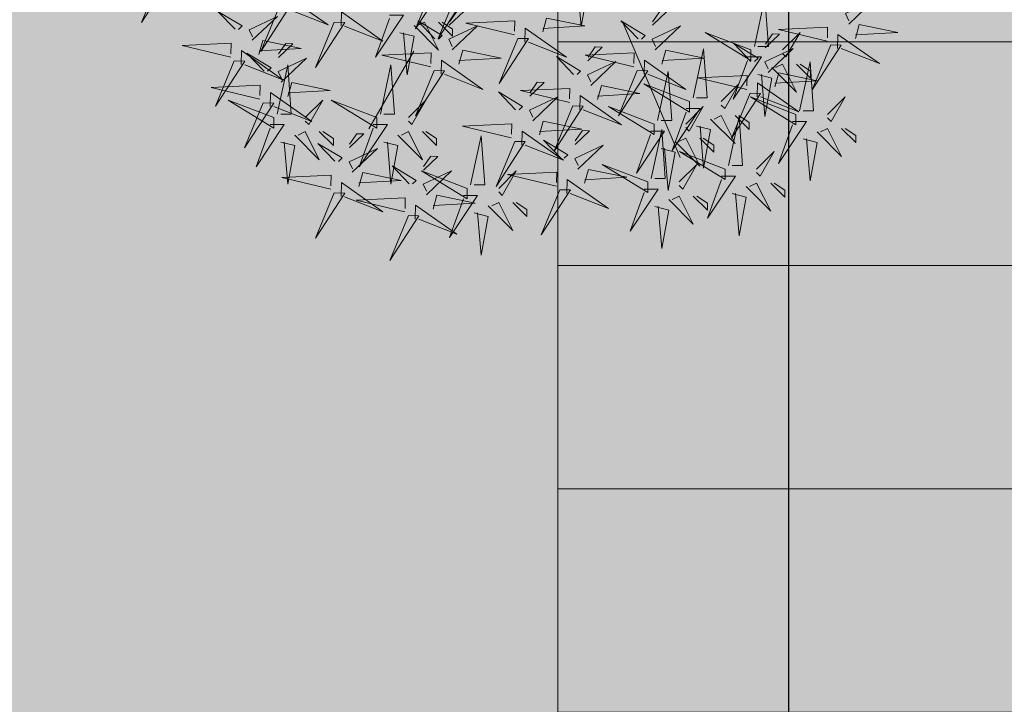
# Model space of a CAD drawing. Units: inches. Extents: x 1704 to 6393, y -157 to 1172.
# Tile 80 of 122: x 2048 to 2081, y 983 to 1006. Entities that reach past the tile are written whole.
import ezdxf

# ---------------------------------------------------------------- set-up
doc = ezdxf.new("R2010")
doc.units = ezdxf.units.IN
doc.header["$MEASUREMENT"] = 0
for name, color, linetype, lineweight in [('A-ANNO-DIMS', 7, 'Continuous', 13), ('L-DECK-PLNK-PATT', 250, 'Continuous', 13), ('L-HRDS', 8, 'Continuous', 18), ('L-shrub', 74, 'Continuous', 18)]:
    doc.layers.add(name, color=color, linetype=linetype, lineweight=lineweight)
doc.layers.add('L-DECK-PATT', color=35, linetype='Continuous', lineweight=13, true_color=0xa6725b)
doc.layers.add('L-HRDS-PATT', color=9, linetype='Continuous', lineweight=13, true_color=0xc5c1ba)
doc.styles.get("Standard").update_dxf_attribs({"font": 'arial.ttf'})
doc.dimstyles.get("Standard").update_dxf_attribs({"dimtxt": 6, "dimasz": 2, "dimexe": 0.18, "dimexo": 0.0625, "dimgap": 0.09, "dimtad": 0, "dimtih": 1, "dimtoh": 1, "dimdec": 1, "dimzin": 0, "dimdsep": 46, "dimlunit": 3, "dimtxsty": 'Standard', "dimblk": 'ARCHTICK', "dimcen": 0.09, "dimadec": 0, "dimazin": 0, "dimtfac": 1, "dimtdec": 1, "dimtofl": 0, "dimtmove": 0, "dimatfit": 3, "dimfxl": 1, "dimtolj": 1, "dimtzin": 0, "dimarcsym": 0})

# ---------------------------------------------------------------- blocks, each defined once
blk = doc.blocks.new('shrub3')
for p, q in [((-68.47, 143.52), (-106.19, 232.32)), ((68.94, 162.35), (98.58, 213.48))]:
    blk.add_line(p, q)
for points in [[(72.58, 270.39), (84.86, 300.11), (65.67, 270.57), (72.58, 270.39)], [(-89.4, 264.53), (-98.64, 266.83), (-94.02, 292.2), (-91.71, 264.53)], [(29.32, 268.76), (20.08, 271.07), (24.7, 296.43), (27.01, 268.76)], [(36.24, 257.23), (27.01, 257.23), (45.48, 284.9), (36.24, 259.54)], [(121.34, 255.57), (133.62, 285.29), (114.43, 255.75), (121.34, 255.57)], [(-140.28, 256.06), (-149.52, 258.36), (-144.9, 283.73), (-142.59, 256.06)], [(-82.48, 253), (-91.71, 253), (-73.24, 280.67), (-82.48, 255.31)], [(-27.06, 253.45), (-14.78, 283.17), (-33.97, 253.63), (-27.06, 253.45)], [(20.08, 264.15), (3.92, 280.29), (13.16, 261.85), (17.78, 264.15)], [(68.03, 272.82), (67.8, 263.59), (40.6, 282.74), (65.73, 272.87)], [(-133.36, 244.53), (-142.59, 244.53), (-124.12, 272.2), (-133.36, 246.84)], [(-98.64, 259.92), (-114.8, 276.06), (-105.56, 257.61), (-100.94, 259.92)], [(-149.52, 251.45), (-165.68, 267.59), (-156.44, 249.14), (-151.83, 251.45)], [(-114.8, 257.61), (-124.03, 266.83), (-124.03, 262.22), (-117.11, 257.61)], [(-31.61, 255.88), (-31.84, 246.65), (-59.04, 265.8), (-33.91, 255.94)], [(3.92, 261.85), (-5.31, 271.07), (-5.31, 266.46), (1.62, 261.85)], [(56.33, 266.18), (53.8, 257.01), (28.56, 262.26), (56.27, 263.87)], [(74.83, 268.03), (106.93, 260.3), (74.6, 258.8), (74.77, 265.72)], [(116.79, 258), (116.56, 248.76), (89.36, 267.92), (114.49, 258.05)], [(33.94, 252.62), (63.95, 241.09), (33.94, 259.54), (33.94, 252.62)], [(-165.68, 249.14), (-174.91, 258.36), (-174.91, 253.75), (-167.99, 249.14)], [(-105.56, 248.39), (-117.11, 236.86), (-107.87, 253), (-105.56, 250.69)], [(-93.64, 226.42), (-102.88, 228.72), (-98.26, 254.08), (-95.95, 226.42)], [(-84.78, 248.39), (-54.77, 236.86), (-84.78, 255.31), (-84.78, 248.39)], [(13.16, 252.62), (1.62, 241.09), (10.85, 257.23), (13.16, 254.93)], [(60.71, 256.84), (44.17, 241.08), (62.84, 249.85), (60.65, 254.53)], [(123.59, 253.21), (155.69, 245.48), (123.36, 243.97), (123.53, 250.9)], [(-186.92, 220.06), (-196.16, 222.37), (-191.54, 247.73), (-189.23, 220.06)], [(-135.66, 239.92), (-105.65, 228.39), (-135.66, 246.84), (-135.66, 239.92)], [(-87.09, 246.08), (-94.02, 213.8), (-96.33, 246.08), (-89.4, 246.08)], [(-43.31, 249.24), (-45.84, 240.07), (-71.08, 245.32), (-43.37, 246.93)], [(-24.81, 251.09), (7.29, 243.36), (-25.04, 241.86), (-24.87, 248.78)], [(2.62, 221.69), (14.9, 251.41), (-4.29, 221.87), (2.62, 221.69)], [(31.63, 250.32), (24.7, 218.04), (22.39, 250.32), (29.32, 250.32)], [(72.06, 249.62), (83.3, 237.79), (67.4, 247.43), (69.76, 249.68)], [(105.09, 251.36), (102.56, 242.19), (77.32, 247.44), (105.04, 249.05)], [(88.68, 222.18), (79.44, 224.49), (84.06, 249.85), (86.37, 222.18)], [(156.52, 222.18), (147.29, 224.49), (151.9, 249.85), (154.21, 222.18)], [(-156.44, 239.92), (-167.99, 228.39), (-158.75, 244.53), (-156.44, 242.22)], [(-86.72, 214.89), (-95.95, 214.89), (-77.48, 242.56), (-86.72, 217.19)], [(-38.93, 239.9), (-55.47, 224.14), (-36.8, 232.91), (-38.99, 237.59)], [(62.61, 240.62), (53.16, 231.62), (57.77, 231.51), (62.55, 238.31)], [(109.47, 242.01), (92.93, 226.26), (111.6, 235.03), (109.41, 239.71)], [(-180, 208.53), (-189.23, 208.53), (-170.76, 236.2), (-180, 210.84)], [(-137.97, 237.61), (-144.9, 205.33), (-147.21, 237.61), (-140.28, 237.61)], [(-116.96, 211.59), (-126.2, 213.9), (-121.58, 239.26), (-119.27, 211.59)], [(-102.88, 221.8), (-119.04, 237.94), (-109.8, 219.5), (-105.18, 221.8)], [(-1.93, 224.12), (-2.16, 214.89), (-29.36, 234.04), (-4.23, 224.17)], [(79.44, 217.57), (63.28, 233.71), (72.52, 215.26), (77.14, 217.57)], [(95.61, 210.65), (86.37, 210.65), (104.84, 238.32), (95.61, 212.96)], [(120.82, 234.8), (132.06, 222.97), (116.16, 232.61), (118.52, 234.86)], [(147.29, 217.57), (131.13, 233.71), (140.36, 215.26), (144.98, 217.57)], [(163.45, 210.65), (154.21, 210.65), (172.68, 238.32), (163.45, 212.96)], [(-196.16, 215.45), (-212.32, 231.59), (-203.08, 213.15), (-198.47, 215.45)], [(-119.04, 219.5), (-128.27, 228.72), (-128.27, 224.11), (-121.35, 219.5)], [(-110.04, 200.06), (-119.27, 200.06), (-100.8, 227.73), (-110.04, 202.37)], [(-35.54, 198.4), (-23.26, 228.12), (-42.45, 198.58), (-35.54, 198.4)], [(-27.58, 232.68), (-16.34, 220.86), (-32.24, 230.49), (-29.88, 232.74)], [(-212.32, 213.15), (-221.55, 222.37), (-221.55, 217.76), (-214.63, 213.15)], [(-126.2, 206.98), (-142.36, 223.12), (-133.12, 204.68), (-128.5, 206.98)], [(-37.03, 223.68), (-46.48, 214.68), (-41.87, 214.57), (-37.09, 221.37)], [(63.28, 215.26), (54.05, 224.49), (54.05, 219.87), (60.98, 215.26)], [(111.37, 225.8), (101.92, 216.8), (106.53, 216.68), (111.31, 223.49)], [(131.13, 215.26), (121.89, 224.49), (121.89, 219.87), (128.82, 215.26)], [(167.98, 196.29), (180.26, 226), (161.07, 196.46), (167.98, 196.29)], [(-152.14, 189.93), (-139.86, 219.65), (-159.05, 190.11), (-152.14, 189.93)], [(-142.36, 204.68), (-151.59, 213.9), (-151.59, 209.29), (-144.67, 204.68)], [(-109.8, 210.27), (-121.35, 198.75), (-112.11, 214.89), (-109.8, 212.58)], [(-89.02, 210.27), (-59.01, 198.75), (-89.02, 217.19), (-89.02, 210.27)], [(-13.63, 217.48), (-16.16, 208.31), (-41.4, 213.56), (-13.69, 215.17)], [(4.87, 219.33), (36.97, 211.6), (4.64, 210.1), (4.81, 217.02)], [(-203.08, 203.92), (-214.63, 192.39), (-205.39, 208.53), (-203.08, 206.23)], [(-182.31, 203.92), (-152.29, 192.39), (-182.31, 210.84), (-182.31, 203.92)], [(-91.33, 207.97), (-98.26, 175.69), (-100.57, 207.97), (-93.64, 207.97)], [(-40.09, 200.83), (-40.32, 191.59), (-67.52, 210.75), (-42.39, 200.88)], [(-9.25, 208.13), (-25.79, 192.38), (-7.12, 201.15), (-9.31, 205.83)], [(72.52, 206.04), (60.98, 194.51), (70.21, 210.65), (72.52, 208.35)], [(93.3, 206.04), (123.31, 194.51), (93.3, 212.96), (93.3, 206.04)], [(140.36, 206.04), (128.82, 194.51), (138.05, 210.65), (140.36, 208.35)], [(163.43, 198.71), (163.2, 189.48), (136, 208.63), (161.13, 198.77)], [(161.14, 206.04), (191.15, 194.51), (161.14, 212.96), (161.14, 206.04)], [(-184.61, 201.62), (-191.54, 169.34), (-193.85, 201.62), (-186.92, 201.62)], [(-156.69, 192.36), (-156.92, 183.12), (-184.12, 202.28), (-159, 192.41)], [(-157.24, 177.72), (-166.48, 180.02), (-161.86, 205.38), (-159.55, 177.72)], [(-112.34, 195.45), (-82.33, 183.92), (-112.34, 202.37), (-112.34, 195.45)], [(-77.94, 175.11), (-65.66, 204.83), (-84.85, 175.28), (-77.94, 175.11)], [(2.1, 200.92), (13.34, 189.09), (-2.56, 198.73), (-0.2, 200.98)], [(55.62, 175.11), (67.9, 204.83), (48.71, 175.28), (55.62, 175.11)], [(90.99, 203.73), (84.06, 171.45), (81.75, 203.73), (88.68, 203.73)], [(158.83, 203.73), (151.9, 171.45), (149.59, 203.73), (156.52, 203.73)], [(-133.12, 195.45), (-144.67, 183.92), (-135.43, 200.06), (-133.12, 197.76)], [(-33.29, 196.04), (-1.19, 188.31), (-33.52, 186.81), (-33.35, 193.73)], [(187.06, 168.76), (199.34, 198.47), (180.15, 168.93), (187.06, 168.76)], [(-205.14, 158.17), (-192.86, 187.89), (-212.05, 158.35), (-205.14, 158.17)], [(-166.48, 173.1), (-182.64, 189.24), (-173.4, 170.8), (-168.79, 173.1)], [(-150.32, 166.19), (-159.55, 166.19), (-141.08, 193.86), (-150.32, 168.49)], [(-114.65, 193.15), (-121.58, 160.87), (-123.89, 193.15), (-116.96, 193.15)], [(-51.79, 194.19), (-54.32, 185.02), (-79.56, 190.27), (-51.85, 191.88)], [(-7.35, 191.92), (-16.8, 182.92), (-12.19, 182.81), (-7.41, 189.61)], [(151.73, 192.07), (149.2, 182.9), (123.96, 188.15), (151.68, 189.77)], [(170.23, 193.92), (202.33, 186.19), (170, 184.69), (170.17, 191.61)], [(-168.39, 185.72), (-170.92, 176.55), (-196.16, 181.8), (-168.45, 183.41)], [(-149.89, 187.57), (-117.79, 179.84), (-150.12, 178.34), (-149.95, 185.26)], [(-82.49, 177.53), (-82.72, 168.3), (-109.92, 187.46), (-84.79, 177.59)], [(-47.41, 184.84), (-63.95, 169.09), (-45.28, 177.86), (-47.47, 182.54)], [(0.5, 153.94), (12.78, 183.65), (-6.41, 154.11), (0.5, 153.94)], [(51.07, 177.53), (50.84, 168.3), (23.64, 187.46), (48.77, 177.59)], [(156.11, 182.73), (139.57, 166.97), (158.24, 175.74), (156.05, 180.42)], [(-182.64, 170.8), (-191.87, 180.02), (-191.87, 175.41), (-184.95, 170.8)], [(-164.01, 176.37), (-180.55, 160.62), (-161.88, 169.39), (-164.07, 174.07)], [(-36.06, 177.63), (-24.82, 165.8), (-40.72, 175.44), (-38.36, 177.69)], [(78.08, 150.19), (68.84, 152.49), (73.46, 177.86), (75.77, 150.19)], [(182.51, 171.18), (182.28, 161.95), (155.08, 181.11), (180.21, 171.24)], [(167.46, 175.51), (178.7, 163.69), (162.8, 173.32), (165.16, 175.57)], [(-209.69, 160.6), (-209.92, 151.36), (-237.12, 170.52), (-212, 160.65)], [(-152.66, 169.16), (-141.42, 157.33), (-157.33, 166.97), (-154.96, 169.22)], [(-152.62, 161.57), (-122.61, 150.05), (-152.62, 168.49), (-152.62, 161.57)], [(-94.19, 170.9), (-96.72, 161.73), (-121.96, 166.98), (-94.25, 168.59)], [(-75.69, 172.75), (-43.59, 165.01), (-75.92, 163.51), (-75.75, 170.44)], [(-45.51, 168.63), (-54.96, 159.63), (-50.35, 159.51), (-45.57, 166.32)], [(39.37, 170.9), (36.84, 161.73), (11.6, 166.98), (39.31, 168.59)], [(57.87, 172.75), (89.97, 165.01), (57.64, 163.51), (57.81, 170.44)], [(121.34, 143.35), (133.62, 173.06), (114.43, 143.52), (121.34, 143.35)], [(-173.4, 161.57), (-184.95, 150.05), (-175.71, 166.19), (-173.4, 163.88)], [(-4.05, 156.36), (-4.28, 147.13), (-31.48, 166.28), (-6.35, 156.42)], [(85.01, 138.66), (75.77, 138.66), (94.24, 166.33), (85.01, 140.97)], [(170.81, 164.55), (168.28, 155.37), (143.04, 160.62), (170.76, 162.24)], [(158.01, 166.51), (148.56, 157.51), (153.17, 157.4), (157.96, 164.21)], [(157.38, 132.76), (169.66, 162.48), (150.47, 132.94), (157.38, 132.76)], [(189.31, 166.39), (221.41, 158.66), (189.08, 157.16), (189.25, 164.09)], [(-202.89, 155.81), (-170.79, 148.07), (-203.12, 146.57), (-202.95, 153.5)], [(-162.11, 160.16), (-171.56, 151.16), (-166.95, 151.04), (-162.17, 157.85)], [(-154.93, 159.27), (-161.86, 126.99), (-164.17, 159.27), (-157.24, 159.27)], [(-89.81, 161.55), (-106.35, 145.8), (-87.68, 154.57), (-89.87, 159.24)], [(43.75, 161.55), (27.21, 145.8), (45.88, 154.57), (43.69, 159.24)], [(68.84, 145.58), (52.68, 161.72), (61.92, 143.27), (66.54, 145.58)], [(116.79, 145.77), (116.56, 136.54), (89.36, 155.7), (114.49, 145.83)], [(-221.39, 153.96), (-223.93, 144.79), (-249.17, 150.04), (-221.45, 151.65)], [(-78.46, 154.34), (-67.22, 142.51), (-83.13, 152.15), (-80.76, 154.4)], [(-15.75, 149.73), (-18.28, 140.55), (-43.52, 145.8), (-15.81, 147.42)], [(2.75, 151.57), (34.85, 143.84), (2.52, 142.34), (2.69, 149.26)], [(40.78, 124.29), (53.06, 154.01), (33.87, 124.47), (40.78, 124.29)], [(52.68, 143.27), (43.45, 152.49), (43.45, 147.88), (50.38, 143.27)], [(55.1, 154.34), (66.34, 142.51), (50.44, 152.15), (52.8, 154.4)], [(175.19, 155.2), (158.65, 139.45), (177.32, 148.22), (175.13, 152.89)], [(-217.01, 144.61), (-233.55, 128.86), (-214.88, 137.63), (-217.07, 142.31)], [(-87.91, 145.34), (-97.36, 136.34), (-92.75, 136.22), (-87.97, 143.03)], [(-36.4, 118.43), (-45.64, 120.73), (-41.02, 146.1), (-38.71, 118.43)], [(45.65, 145.34), (36.2, 136.34), (40.81, 136.22), (45.59, 143.03)], [(55.62, 117.94), (67.9, 147.66), (48.71, 118.11), (55.62, 117.94)], [(152.83, 135.19), (152.6, 125.95), (125.4, 145.11), (150.53, 135.24)], [(186.54, 147.99), (197.78, 136.16), (181.88, 145.8), (184.24, 148.05)], [(235.82, 113.71), (248.1, 143.42), (228.91, 113.88), (235.82, 113.71)]]:
    blk.add_lwpolyline(points)
blk = doc.blocks.new('_ArchTick')
at = {"color": 0, "linetype": 'ByBlock', "const_width": 0.15}
blk.add_lwpolyline([(-0.5, -0.5), (0.5, 0.5)], dxfattribs=at)
blk = doc.blocks.new('*D92')
at = {"layer": 'A-ANNO-DIMS', "color": 0, "lineweight": -2, "transparency": 16777216}
for p, q in [((2073.349, 895.275), (2073.349, 1105.287)), ((2073.349, 1105.107), (2332.661, 1105.107)), ((2605.349, 1105.107), (2346.036, 1105.107)), ((2605.349, 895.275), (2605.349, 1105.287))]:
    blk.add_line(p, q, dxfattribs=at)
at = {"layer": 'Defpoints', "color": 0, "lineweight": -3, "transparency": 16777216}
for p in [(2605.349, 1105.107), (2073.349, 895.213), (2605.349, 895.213)]:
    blk.add_point(p, dxfattribs=at)
at = {"layer": 'A-ANNO-DIMS', "color": 0, "lineweight": -2, "transparency": 16777216, "xscale": 2, "yscale": 2, "zscale": 2, "rotation": 180}
blk.add_blockref('_ArchTick', (2073.349, 1105.107), dxfattribs=at)
at = {"layer": 'A-ANNO-DIMS', "color": 0, "lineweight": -2, "transparency": 16777216, "xscale": 2, "yscale": 2, "zscale": 2}
blk.add_blockref('_ArchTick', (2605.349, 1105.107), dxfattribs=at)
at = {"layer": 'A-ANNO-DIMS', "color": 0, "transparency": 16777216, "insert": (2339.349, 1105.107), "char_height": 6, "attachment_point": 5}
blk.add_mtext('\\A1;532', dxfattribs=at)
blk = doc.blocks.new('*D94')
at = {"layer": 'A-ANNO-DIMS', "color": 0, "lineweight": -2, "transparency": 16777216}
for p, q in [((1898.349, 895.275), (1898.349, 1105.287)), ((1898.349, 1105.107), (1979.39, 1105.107)), ((2073.349, 1105.107), (1992.307, 1105.107)), ((2073.349, 895.275), (2073.349, 1105.287))]:
    blk.add_line(p, q, dxfattribs=at)
at = {"layer": 'Defpoints', "color": 0, "lineweight": -3, "transparency": 16777216}
for p in [(2073.349, 1105.107), (1898.349, 895.213), (2073.349, 895.213)]:
    blk.add_point(p, dxfattribs=at)
at = {"layer": 'A-ANNO-DIMS', "color": 0, "lineweight": -2, "transparency": 16777216, "xscale": 2, "yscale": 2, "zscale": 2, "rotation": 180}
blk.add_blockref('_ArchTick', (1898.349, 1105.107), dxfattribs=at)
at = {"layer": 'A-ANNO-DIMS', "color": 0, "lineweight": -2, "transparency": 16777216, "xscale": 2, "yscale": 2, "zscale": 2}
blk.add_blockref('_ArchTick', (2073.349, 1105.107), dxfattribs=at)
at = {"layer": 'A-ANNO-DIMS', "color": 0, "transparency": 16777216, "insert": (1985.849, 1105.107), "char_height": 6, "attachment_point": 5}
blk.add_mtext('\\A1;175', dxfattribs=at)

msp = doc.modelspace()

# ---------------------------------------------------------------- hatches: boundary and pattern name
at = {"layer": 'L-DECK-PATT', "transparency": 33554544}
h = msp.add_hatch(color=256, dxfattribs=at)
h.dxf.hatch_style = 1
h.paths.add_polyline_path([(2329.589, 1033.213), (2065.589, 1033.213), (2065.589, 895.213), (2167.349, 895.213), (2263.349, 895.213), (2263.349, 903.213), (2273.349, 903.213), (2273.349, 895.213), (2329.589, 895.213)])
h.paths.add_polyline_path([(2664.349, 1033.213), (2333.589, 1033.213), (2333.589, 895.213), (2465.349, 895.213), (2469.181, 895.213), (2470.482, 895.213), (2508.215, 895.213), (2509.516, 895.213), (2513.349, 895.213), (2533.349, 895.213), (2581.349, 895.213), (2605.349, 895.213), (2664.349, 895.213)])
h.paths.add_polyline_path([(2333.589, 1033.213), (2329.589, 1033.213), (2329.589, 895.213), (2333.589, 895.213)])
at = {"layer": 'L-DECK-PLNK-PATT'}
h = msp.add_hatch(dxfattribs=at)
h.set_pattern_fill('LINE', color=256, scale=60)
h.paths.add_polyline_path([(2329.589, 1033.213), (2065.589, 1033.213), (2065.589, 895.213), (2167.349, 895.213), (2263.349, 895.213), (2263.349, 903.213), (2273.349, 903.213), (2273.349, 895.213), (2329.589, 895.213)])
h.paths.add_polyline_path([(2664.349, 1033.213), (2333.589, 1033.213), (2333.589, 895.213), (2465.349, 895.213), (2469.181, 895.213), (2470.482, 895.213), (2508.215, 895.213), (2509.516, 895.213), (2513.349, 895.213), (2533.349, 895.213), (2581.349, 895.213), (2605.349, 895.213), (2664.349, 895.213)])
h.paths.add_polyline_path([(2333.589, 1033.213), (2329.589, 1033.213), (2329.589, 895.213), (2333.589, 895.213)])
at = {"layer": 'L-HRDS-PATT', "transparency": 33554643}
h = msp.add_hatch(color=256, dxfattribs=at)
h.dxf.hatch_style = 1
h.paths.add_polyline_path([(2065.589, 1033.213), (1898.349, 1033.213), (1898.349, 895.213), (2065.589, 895.213)])

# ---------------------------------------------------------------- linework, layer by layer
at = {"layer": 'L-HRDS'}
msp.add_line((2065.589, 895.213), (2065.589, 1033.213), dxfattribs=at)

# ---------------------------------------------------------------- block references
at = {"layer": 'L-shrub', "xscale": 0.0510581485411622, "yscale": 0.0510581485411622, "zscale": 0.0510581485411622, "rotation": 180}
msp.add_blockref('shrub3', (2064.28, 1012.986), dxfattribs=at)

# ---------------------------------------------------------------- dimensions: what is measured, and where the dimension line sits
at = {"layer": 'A-ANNO-DIMS'}
for base, p1, p2, picture, middle in [((2073.349, 1105.107), (1898.349, 895.213), (2073.349, 895.213), '*D94', (1985.849, 1105.107)), ((2605.349, 1105.107), (2073.349, 895.213), (2605.349, 895.213), '*D92', (2339.349, 1105.107))]:
    dim = msp.add_linear_dim(base=base, p1=p1, p2=p2, dimstyle='Standard', override={"dimdec": 0, "dimlfac": 1, "dimrnd": 0, "dimzin": 0, "dimdsep": 46, "dimlunit": 2}, dxfattribs=at)
    dim.commit()
    dim.dimension.update_dxf_attribs({"geometry": picture, "text_midpoint": middle})

doc.saveas('drawing.dxf')
